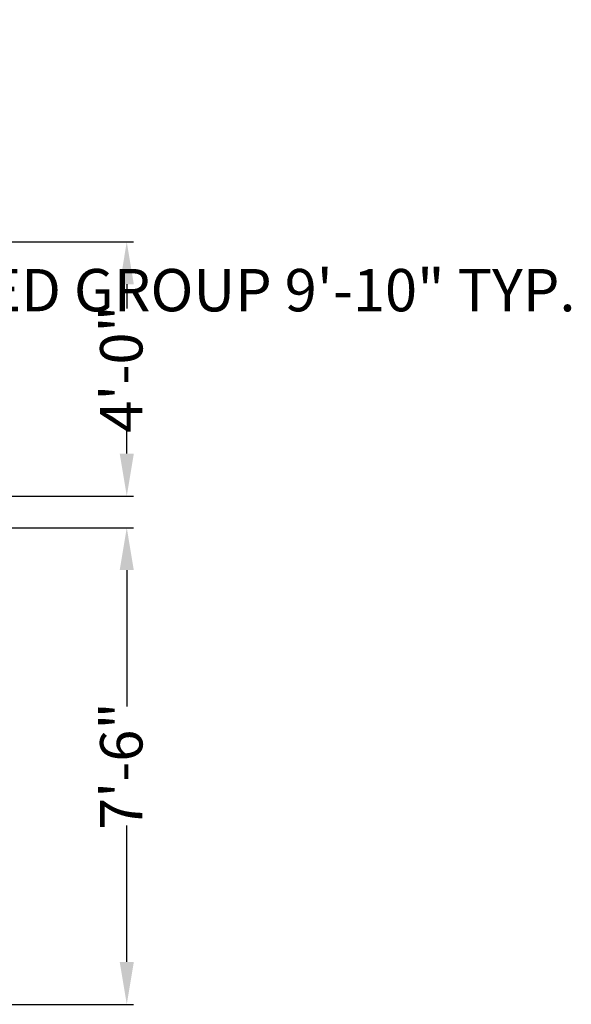
# Model space of a CAD drawing. Units: inches. Extents: x 2073 to 2646, y 2372 to 3017.
# Tile 7 of 8: x 2542 to 2646, y 2688 to 2874. Entities that reach past the tile are written whole.
import ezdxf

# ---------------------------------------------------------------- set-up
doc = ezdxf.new("R2010")
doc.units = ezdxf.units.IN
doc.layers.add('A-ANNO-DIMS', color=2, linetype='Continuous', lineweight=18)
doc.styles.get("Standard").update_dxf_attribs({"font": 'arial.ttf'})
doc.dimstyles.new('ISO-25', dxfattribs={"dimtxt": 8, "dimasz": 8, "dimexe": 1.25, "dimexo": 0.625, "dimtad": 0, "dimdec": 1, "dimlunit": 4, "dimtxsty": 'Standard', "dimcen": 2.5, "dimadec": 0, "dimazin": 0, "dimtfac": 1, "dimtdec": 1, "dimtmove": 0, "dimatfit": 3, "dimfxl": 1, "dimarcsym": 0})

# ---------------------------------------------------------------- blocks, each defined once
blk = doc.blocks.new('*D35')
at = {"layer": 'A-ANNO-DIMS', "color": 0, "lineweight": -2, "transparency": 16777216}
for p, q in [((2398.23, 2838.6), (2398.23, 2820.25)), ((2516.35, 2838.6), (2516.35, 2820.25)), ((2406.23, 2821.5), (2508.35, 2821.5)), ((2516.35, 2821.5), (2524.35, 2821.5))]:
    blk.add_line(p, q, dxfattribs=at)
at = {"layer": 'A-ANNO-DIMS', "color": 0, "transparency": 16777216}
for points in [[(2406.23, 2822.84), (2406.23, 2820.17), (2398.23, 2821.5)], [(2508.35, 2822.84), (2508.35, 2820.17), (2516.35, 2821.5)]]:
    blk.add_solid(points, dxfattribs=at)
at = {"layer": 'Defpoints', "color": 0, "transparency": 16777216}
for p in [(2398.23, 2839.22), (2516.35, 2839.22), (2516.35, 2821.5)]:
    blk.add_point(p, dxfattribs=at)
at = {"layer": 'A-ANNO-DIMS', "color": 0, "transparency": 16777216, "insert": (2587.37, 2821.5), "char_height": 8, "attachment_point": 5}
blk.add_mtext('BED GROUP 9\'-10" TYP.', dxfattribs=at)
blk = doc.blocks.new('*D36')
at = {"layer": 'A-ANNO-DIMS', "color": 0, "lineweight": -2, "transparency": 16777216}
for p, q in [((2516.97, 2939.66), (2535.31, 2939.66)), ((2534.06, 2931.66), (2534.06, 2923.78)), ((2534.06, 2847.22), (2534.06, 2855.11)), ((2516.97, 2839.22), (2535.31, 2839.22))]:
    blk.add_line(p, q, dxfattribs=at)
at = {"layer": 'A-ANNO-DIMS', "color": 0, "transparency": 16777216}
for points in [[(2532.73, 2931.66), (2535.39, 2931.66), (2534.06, 2939.66)], [(2532.73, 2847.22), (2535.39, 2847.22), (2534.06, 2839.22)]]:
    blk.add_solid(points, dxfattribs=at)
at = {"layer": 'Defpoints', "color": 0, "transparency": 16777216}
for p in [(2516.35, 2939.66), (2534.06, 2939.66), (2516.35, 2839.22)]:
    blk.add_point(p, dxfattribs=at)
at = {"layer": 'A-ANNO-DIMS', "color": 0, "transparency": 16777216, "insert": (2534.06, 2889.44), "char_height": 8, "attachment_point": 5, "rotation": 90}
blk.add_mtext('8\'-4 1/2" TYP.', dxfattribs=at)
blk = doc.blocks.new('*D45')
at = {"layer": 'A-ANNO-DIMS', "color": 0, "lineweight": -2, "transparency": 16777216}
for p, q in [((2523.92, 2777.66), (2563.04, 2777.66)), ((2561.79, 2769.66), (2561.79, 2743.89)), ((2561.79, 2695.66), (2561.79, 2721.44)), ((2523.92, 2687.66), (2563.04, 2687.66))]:
    blk.add_line(p, q, dxfattribs=at)
at = {"layer": 'A-ANNO-DIMS', "color": 0, "transparency": 16777216}
for points in [[(2560.46, 2769.66), (2563.12, 2769.66), (2561.79, 2777.66)], [(2560.46, 2695.66), (2563.12, 2695.66), (2561.79, 2687.66)]]:
    blk.add_solid(points, dxfattribs=at)
at = {"layer": 'Defpoints', "color": 0, "transparency": 16777216}
for p in [(2523.29, 2777.66), (2561.79, 2777.66), (2523.29, 2687.66)]:
    blk.add_point(p, dxfattribs=at)
at = {"layer": 'A-ANNO-DIMS', "color": 0, "transparency": 16777216, "insert": (2561.79, 2732.66), "char_height": 8, "attachment_point": 5, "rotation": 90}
blk.add_mtext('7\'-6"', dxfattribs=at)
blk = doc.blocks.new('*D56')
at = {"layer": 'A-ANNO-DIMS', "color": 0, "lineweight": -2, "transparency": 16777216}
for p, q in [((2523.92, 2831.66), (2563.04, 2831.66)), ((2561.79, 2823.66), (2561.79, 2819.08)), ((2561.79, 2791.66), (2561.79, 2796.25)), ((2523.92, 2783.66), (2563.04, 2783.66))]:
    blk.add_line(p, q, dxfattribs=at)
at = {"layer": 'A-ANNO-DIMS', "color": 0, "transparency": 16777216}
for points in [[(2560.46, 2823.66), (2563.12, 2823.66), (2561.79, 2831.66)], [(2560.46, 2791.66), (2563.12, 2791.66), (2561.79, 2783.66)]]:
    blk.add_solid(points, dxfattribs=at)
at = {"layer": 'Defpoints', "color": 0, "transparency": 16777216}
for p in [(2523.29, 2831.66), (2561.79, 2831.66), (2523.29, 2783.66)]:
    blk.add_point(p, dxfattribs=at)
at = {"layer": 'A-ANNO-DIMS', "color": 0, "transparency": 16777216, "insert": (2561.79, 2807.66), "char_height": 8, "attachment_point": 5, "rotation": 90}
blk.add_mtext('4\'-0"', dxfattribs=at)

msp = doc.modelspace()

# ---------------------------------------------------------------- dimensions: what is measured, and where the dimension line sits
at = {"layer": 'A-ANNO-DIMS'}
dim = msp.add_linear_dim(base=(2534.06, 2939.66), p1=(2516.35, 2839.22), p2=(2516.35, 2939.66), angle=90, text='<> TYP.', dimstyle='ISO-25', override={"dimdec": 1, "dimlfac": 1, "dimrnd": 0, "dimzin": 1, "dimdsep": 46, "dimlunit": 4, "dimfrac": 2}, dxfattribs=at)
dim.commit()
dim.dimension.update_dxf_attribs({"geometry": '*D36', "text_midpoint": (2534.06, 2889.44)})
dim = msp.add_linear_dim(base=(2516.35, 2821.5), p1=(2398.23, 2839.22), p2=(2516.35, 2839.22), text='BED GROUP <> TYP.', dimstyle='ISO-25', override={"dimdec": 1, "dimlfac": 1, "dimrnd": 0, "dimzin": 1, "dimdsep": 46, "dimlunit": 4, "dimfrac": 2}, dxfattribs=at)
dim.commit()
dim.dimension.update_dxf_attribs({"geometry": '*D35', "text_midpoint": (2587.37, 2821.5)})
for base, p1, p2, picture, middle in [((2561.79, 2831.66), (2523.29, 2783.66), (2523.29, 2831.66), '*D56', (2561.79, 2807.66)), ((2561.79, 2777.66), (2523.29, 2687.66), (2523.29, 2777.66), '*D45', (2561.79, 2732.66))]:
    dim = msp.add_linear_dim(base=base, p1=p1, p2=p2, angle=90, dimstyle='ISO-25', override={"dimdec": 1, "dimlfac": 1, "dimrnd": 0, "dimzin": 1, "dimdsep": 46, "dimlunit": 4, "dimfrac": 2}, dxfattribs=at)
    dim.commit()
    dim.dimension.update_dxf_attribs({"geometry": picture, "text_midpoint": middle})

doc.saveas('drawing.dxf')
